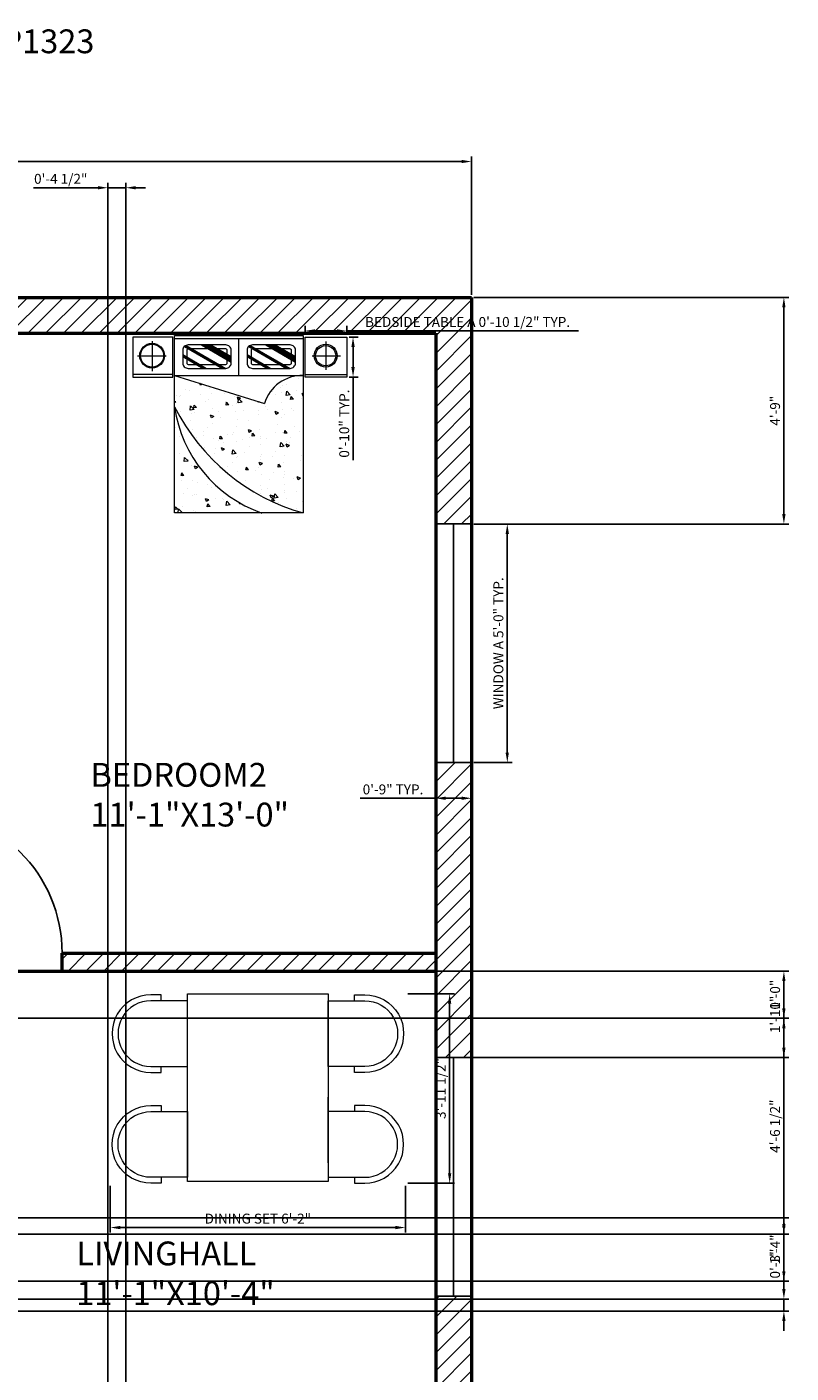
# Model space of a CAD drawing. Units: inches. Extents: x 3064 to 3516, y 2736 to 3280.
# Tile 5 of 5: x 3324 to 3516, y 2941 to 3280. Entities that reach past the tile are written whole.
import ezdxf

# ---------------------------------------------------------------- set-up
doc = ezdxf.new("R2010")
doc.units = ezdxf.units.IN
for name, color, linetype, lineweight in [('A-ANNO-DIMS', 2, 'Continuous', 18), ('A-ANNO-TEXT', 7, 'Continuous', 25), ('A-AREA-IDEN', 6, 'Continuous', 25), ('A-DOOR', 3, 'Continuous', 25), ('A-FURN', 8, 'Continuous', 18), ('A-FURN-PATT', 9, 'Continuous', 13), ('A-GLAZ', 5, 'Continuous', 25), ('A-WALL', 7, 'Continuous', 50), ('A-WALL-PATT', 8, 'Continuous', 13)]:
    doc.layers.add(name, color=color, linetype=linetype, lineweight=lineweight)
doc.styles.get("Standard").update_dxf_attribs({"font": 'arial.ttf'})
doc.dimstyles.new('ISO-25', dxfattribs={"dimtxt": 2.5, "dimasz": 2.5, "dimexe": 1.25, "dimexo": 0.625, "dimtad": 1, "dimlunit": 3, "dimtxsty": 'Standard', "dimcen": 2.5, "dimadec": 0, "dimazin": 0, "dimtfac": 1, "dimtmove": 0, "dimatfit": 3, "dimfxl": 1, "dimarcsym": 0})

# ---------------------------------------------------------------- blocks, each defined once
blk = doc.blocks.new('*D3')
at = {"layer": 'A-ANNO-DIMS', "color": 0, "lineweight": -2, "transparency": 16777216}
for p, q in [((3147.2, 3213.35), (3147.2, 3246.96)), ((3149.7, 3245.71), (3432.9, 3245.71)), ((3435.4, 3212.14), (3435.4, 3246.96))]:
    blk.add_line(p, q, dxfattribs=at)
at = {"layer": 'A-ANNO-DIMS', "color": 0, "transparency": 16777216}
for points in [[(3149.7, 3246.13), (3149.7, 3245.3), (3147.2, 3245.71)], [(3432.9, 3246.13), (3432.9, 3245.3), (3435.4, 3245.71)]]:
    blk.add_solid(points, dxfattribs=at)
at = {"layer": 'Defpoints', "color": 0, "transparency": 16777216}
for p in [(3435.4, 3245.71), (3147.2, 3212.72), (3435.4, 3211.51)]:
    blk.add_point(p, dxfattribs=at)
at = {"layer": 'A-ANNO-DIMS', "color": 0, "transparency": 16777216, "insert": (3291.3, 3249.4), "char_height": 6, "attachment_point": 5}
blk.add_mtext('24\'-0.2"', dxfattribs=at)
blk = doc.blocks.new('4 Person Square 02')
for p, q in [((450, 1104.5), (450, 683.9)), ((-450, 119.2), (-450, 539.9)), ((450, 119.2), (450, 539.9)), ((450, 119.2), (450, 539.9))]:
    blk.add_line(p, q)
for points in [[(-617.2, 1155.3), (-617.2, 1193.5), (-683.2, 1193.5, 1.001343), (-683.2, 697), (-617.2, 697), (-617.2, 735.3)], [(617.2, 1155.3), (617.2, 1193.5), (683.2, 1193.5, -1.001343), (683.2, 697), (617.2, 697), (617.2, 735.3)], [(-617.2, 27.3), (-617.2, -10.9), (-683.2, -10.9, -1.001343), (-683.2, 485.6), (-617.2, 485.6), (-617.2, 447.3)], [(617.2, 27.3), (617.2, -10.9), (683.2, -10.9, 1.001343), (683.2, 485.6), (617.2, 485.6), (617.2, 447.3)]]:
    blk.add_lwpolyline(points, format="xyb")
for points in [[(-450, 735.3), (-450, 1155.3), (-617.2, 1155.3), (-683.2, 1155.3, 1.001587), (-683.2, 735.3)], [(450, 735.3), (450, 1155.3), (617.2, 1155.3), (683.2, 1155.3, -1.001587), (683.2, 735.3)], [(-450, 447.3), (-450, 27.3), (-617.2, 27.3), (-683.2, 27.3, -1.001587), (-683.2, 447.3)], [(450, 447.3), (450, 27.3), (617.2, 27.3), (683.2, 27.3, 1.001587), (683.2, 447.3)]]:
    blk.add_lwpolyline(points, format="xyb", close=True)
blk.add_lwpolyline([(450, 0), (-450, 0), (-450, 1200), (450, 1200)], close=True)
blk = doc.blocks.new('DOOR-SWING-36IN')
for p, q in [((-1, -4.5), (-1, 36)), ((0, 0), (0, 36))]:
    blk.add_line(p, q)
blk.add_arc((0, 0), 36, 90, 180)
blk = doc.blocks.new('WIN-60IN')
for p, q in [((0, 60), (0, 0)), ((9, 60), (0, 60)), ((4.5, 60), (4.5, 0)), ((9, 0), (9, 60)), ((0, 0), (9, 0))]:
    blk.add_line(p, q)
blk = doc.blocks.new('BEDSIDE-TABLE-A')
for p, q in [((0, 0), (0, 10.49)), ((0, 10.49), (10.04, 10.49)), ((9.38, 0), (9.38, 10.49)), ((10.04, 10.49), (10.04, 0)), ((4.67, 1.81), (4.67, 8.9)), ((1.1, 5.18), (8.23, 5.18)), ((10.04, 0), (0, 0))]:
    blk.add_line(p, q)
for radius in [2.89, 2.54]:
    blk.add_circle((4.67, 5.18), radius)
blk = doc.blocks.new('BEDSIDE-TABLE-B')
for p, q in [((10.04, 10.04), (0, 10.04)), ((0, 10.04), (0, 0)), ((4.67, 1.21), (4.67, 8.43)), ((9.34, 0), (9.34, 10.04)), ((10.04, 0), (10.04, 10.04)), ((1.04, 4.86), (8.55, 4.86)), ((0, 0), (10.04, 0))]:
    blk.add_line(p, q)
for radius in [3.11, 2.89]:
    blk.add_circle((4.67, 4.86), radius)
blk = doc.blocks.new('BED-FRAME-AND-COVER')
for p, q in [((0, 32.36), (44.63, 32.36)), ((0, 0), (0, 32.36)), ((0.73, 0), (0.73, 32.36)), ((10.02, 0), (10.02, 32.36)), ((44.63, 32.36), (44.63, 0)), ((10.02, 0), (17.09, 22.61)), ((10.02, 16.18), (0.73, 16.18)), ((44.63, 0), (0, 0))]:
    blk.add_line(p, q)
for centre, radius, start, end in [((20, 32.16), 9.98, 178.8468, 253.0453), ((-5.57, 46.57), 52.17, 296.7955, 344.1914), ((13.16, 33.03), 33.38, 278.2583, 340.5572)]:
    blk.add_arc(centre, radius, start, end)
blk = doc.blocks.new('*D19')
at = {"layer": 'A-ANNO-DIMS', "color": 0, "lineweight": -2, "transparency": 16777216}
for p, q in [((3436.02, 3154.51), (3445.65, 3154.51)), ((3444.4, 3152.01), (3444.4, 3097.01)), ((3436.02, 3094.51), (3445.65, 3094.51))]:
    blk.add_line(p, q, dxfattribs=at)
at = {"layer": 'A-ANNO-DIMS', "color": 0, "transparency": 16777216}
for points in [[(3443.98, 3152.01), (3444.81, 3152.01), (3444.4, 3154.51)], [(3443.98, 3097.01), (3444.81, 3097.01), (3444.4, 3094.51)]]:
    blk.add_solid(points, dxfattribs=at)
at = {"layer": 'Defpoints', "color": 0, "transparency": 16777216}
for p in [(3435.4, 3154.51), (3435.4, 3094.51), (3444.4, 3094.51)]:
    blk.add_point(p, dxfattribs=at)
at = {"layer": 'A-ANNO-DIMS', "color": 0, "transparency": 16777216, "insert": (3442.48, 3124.51), "char_height": 2.5, "attachment_point": 5, "rotation": 90}
blk.add_mtext('WINDOW A 5\'-0" TYP.', dxfattribs=at)
blk = doc.blocks.new('*D20')
at = {"layer": 'A-ANNO-DIMS', "color": 0, "lineweight": -2, "transparency": 16777216}
for p, q in [((3426.4, 3093.89), (3426.4, 3084.26)), ((3435.4, 3093.89), (3435.4, 3084.26)), ((3426.4, 3085.51), (3407.41, 3085.51)), ((3432.9, 3085.51), (3428.9, 3085.51))]:
    blk.add_line(p, q, dxfattribs=at)
at = {"layer": 'A-ANNO-DIMS', "color": 0, "transparency": 16777216}
for points in [[(3428.9, 3085.93), (3428.9, 3085.1), (3426.4, 3085.51)], [(3432.9, 3085.93), (3432.9, 3085.1), (3435.4, 3085.51)]]:
    blk.add_solid(points, dxfattribs=at)
at = {"layer": 'Defpoints', "color": 0, "transparency": 16777216}
for p in [(3426.4, 3094.51), (3435.4, 3094.51), (3426.4, 3085.51)]:
    blk.add_point(p, dxfattribs=at)
at = {"layer": 'A-ANNO-DIMS', "color": 0, "transparency": 16777216, "insert": (3415.65, 3087.42), "char_height": 2.5, "attachment_point": 5}
blk.add_mtext('0\'-9" TYP.', dxfattribs=at)
blk = doc.blocks.new('*D25')
at = {"layer": 'A-ANNO-DIMS', "color": 0, "lineweight": -2, "transparency": 16777216}
for p, q in [((3393.53, 3202.15), (3393.53, 3204.35)), ((3404.02, 3202.15), (3404.02, 3204.35)), ((3396.03, 3203.1), (3401.52, 3203.1)), ((3404.02, 3203.1), (3462.3, 3203.1))]:
    blk.add_line(p, q, dxfattribs=at)
at = {"layer": 'A-ANNO-DIMS', "color": 0, "transparency": 16777216}
for points in [[(3396.03, 3203.51), (3396.03, 3202.68), (3393.53, 3203.1)], [(3401.52, 3203.51), (3401.52, 3202.68), (3404.02, 3203.1)]]:
    blk.add_solid(points, dxfattribs=at)
at = {"layer": 'Defpoints', "color": 0, "transparency": 16777216}
for p in [(3393.53, 3201.52), (3404.02, 3203.1), (3404.02, 3201.52)]:
    blk.add_point(p, dxfattribs=at)
at = {"layer": 'A-ANNO-DIMS', "color": 0, "transparency": 16777216, "insert": (3434.41, 3205.02), "char_height": 2.5, "attachment_point": 5}
blk.add_mtext('BEDSIDE TABLE A 0\'-10 1/2" TYP.', dxfattribs=at)
blk = doc.blocks.new('*D26')
at = {"layer": 'A-ANNO-DIMS', "color": 0, "lineweight": -2, "transparency": 16777216}
for p, q in [((3404.64, 3201.52), (3406.84, 3201.52)), ((3405.59, 3199.02), (3405.59, 3193.98)), ((3404.64, 3191.48), (3406.84, 3191.48)), ((3405.59, 3191.48), (3405.59, 3170.55))]:
    blk.add_line(p, q, dxfattribs=at)
at = {"layer": 'A-ANNO-DIMS', "color": 0, "transparency": 16777216}
for points in [[(3405.17, 3199.02), (3406.01, 3199.02), (3405.59, 3201.52)], [(3405.17, 3193.98), (3406.01, 3193.98), (3405.59, 3191.48)]]:
    blk.add_solid(points, dxfattribs=at)
at = {"layer": 'Defpoints', "color": 0, "transparency": 16777216}
for p in [(3404.02, 3201.52), (3404.02, 3191.48), (3405.59, 3191.48)]:
    blk.add_point(p, dxfattribs=at)
at = {"layer": 'A-ANNO-DIMS', "color": 0, "transparency": 16777216, "insert": (3403.69, 3179.77), "char_height": 2.5, "attachment_point": 5, "rotation": 90}
blk.add_mtext('0\'-10" TYP.', dxfattribs=at)
blk = doc.blocks.new('*D35')
at = {"layer": 'A-ANNO-DIMS', "color": 0, "lineweight": -2, "transparency": 16777216}
for p, q in [((3344.51, 2988.02), (3344.51, 2976.26)), ((3418.76, 2988.02), (3418.76, 2976.26)), ((3347.01, 2977.51), (3416.26, 2977.51))]:
    blk.add_line(p, q, dxfattribs=at)
at = {"layer": 'A-ANNO-DIMS', "color": 0, "transparency": 16777216}
for points in [[(3347.01, 2977.93), (3347.01, 2977.09), (3344.51, 2977.51)], [(3416.26, 2977.93), (3416.26, 2977.09), (3418.76, 2977.51)]]:
    blk.add_solid(points, dxfattribs=at)
at = {"layer": 'Defpoints', "color": 0, "transparency": 16777216}
for p in [(3344.51, 2988.65), (3418.76, 2988.65), (3418.76, 2977.51)]:
    blk.add_point(p, dxfattribs=at)
at = {"layer": 'A-ANNO-DIMS', "color": 0, "transparency": 16777216, "insert": (3381.64, 2979.43), "char_height": 2.5, "attachment_point": 5}
blk.add_mtext('DINING SET 6\'-2"', dxfattribs=at)
blk = doc.blocks.new('*D36')
at = {"layer": 'A-ANNO-DIMS', "color": 0, "lineweight": -2, "transparency": 16777216}
for p, q in [((3419.38, 3036.32), (3431.15, 3036.32)), ((3429.9, 2991.15), (3429.9, 3033.82)), ((3419.38, 2988.65), (3431.15, 2988.65))]:
    blk.add_line(p, q, dxfattribs=at)
at = {"layer": 'A-ANNO-DIMS', "color": 0, "transparency": 16777216}
for points in [[(3429.48, 3033.82), (3430.31, 3033.82), (3429.9, 3036.32)], [(3429.48, 2991.15), (3430.31, 2991.15), (3429.9, 2988.65)]]:
    blk.add_solid(points, dxfattribs=at)
at = {"layer": 'Defpoints', "color": 0, "transparency": 16777216}
for p in [(3418.76, 3036.32), (3429.9, 3036.32), (3418.76, 2988.65)]:
    blk.add_point(p, dxfattribs=at)
at = {"layer": 'A-ANNO-DIMS', "color": 0, "transparency": 16777216, "insert": (3427.98, 3012.49), "char_height": 2.5, "attachment_point": 5, "rotation": 90}
blk.add_mtext('3\'-11 1/2"', dxfattribs=at)
blk = doc.blocks.new('*D41')
at = {"layer": 'A-ANNO-DIMS', "color": 0, "lineweight": -2, "transparency": 16777216}
for p, q in [((3427.02, 3042.01), (3515.25, 3042.01)), ((3514, 3022.76), (3514, 3039.51)), ((3427.02, 3020.26), (3515.25, 3020.26))]:
    blk.add_line(p, q, dxfattribs=at)
at = {"layer": 'A-ANNO-DIMS', "color": 0, "transparency": 16777216}
for points in [[(3513.58, 3039.51), (3514.41, 3039.51), (3514, 3042.01)], [(3513.58, 3022.76), (3514.41, 3022.76), (3514, 3020.26)]]:
    blk.add_solid(points, dxfattribs=at)
at = {"layer": 'Defpoints', "color": 0, "transparency": 16777216}
for p in [(3426.4, 3042.01), (3514, 3042.01), (3426.4, 3020.26)]:
    blk.add_point(p, dxfattribs=at)
at = {"layer": 'A-ANNO-DIMS', "color": 0, "transparency": 16777216, "insert": (3512.1, 3031.14), "char_height": 2.5, "attachment_point": 5, "rotation": 90}
blk.add_mtext('1\'-10"', dxfattribs=at)
blk = doc.blocks.new('*D42')
at = {"layer": 'A-ANNO-DIMS', "color": 0, "lineweight": -2, "transparency": 16777216}
for p, q in [((3436.02, 3211.51), (3515.25, 3211.51)), ((3514, 3157.01), (3514, 3209.01)), ((3436.02, 3154.51), (3515.25, 3154.51))]:
    blk.add_line(p, q, dxfattribs=at)
at = {"layer": 'A-ANNO-DIMS', "color": 0, "transparency": 16777216}
for points in [[(3513.58, 3209.01), (3514.41, 3209.01), (3514, 3211.51)], [(3513.58, 3157.01), (3514.41, 3157.01), (3514, 3154.51)]]:
    blk.add_solid(points, dxfattribs=at)
at = {"layer": 'Defpoints', "color": 0, "transparency": 16777216}
for p in [(3435.4, 3211.51), (3514, 3211.51), (3435.4, 3154.51)]:
    blk.add_point(p, dxfattribs=at)
at = {"layer": 'A-ANNO-DIMS', "color": 0, "transparency": 16777216, "insert": (3512.1, 3183.01), "char_height": 2.5, "attachment_point": 5, "rotation": 90}
blk.add_mtext('4\'-9"', dxfattribs=at)
blk = doc.blocks.new('*D44')
at = {"layer": 'A-ANNO-DIMS', "color": 0, "lineweight": -2, "transparency": 16777216}
for p, q in [((3341.4, 3239.11), (3325.18, 3239.11)), ((3343.9, 2921.14), (3343.9, 3240.36)), ((3348.4, 3239.11), (3343.9, 3239.11)), ((3348.4, 2921.14), (3348.4, 3240.36)), ((3350.9, 3239.11), (3353.4, 3239.11))]:
    blk.add_line(p, q, dxfattribs=at)
at = {"layer": 'A-ANNO-DIMS', "color": 0, "transparency": 16777216}
for points in [[(3341.4, 3239.53), (3341.4, 3238.7), (3343.9, 3239.11)], [(3350.9, 3239.53), (3350.9, 3238.7), (3348.4, 3239.11)]]:
    blk.add_solid(points, dxfattribs=at)
at = {"layer": 'Defpoints', "color": 0, "transparency": 16777216}
for p in [(3343.9, 3239.11), (3343.9, 2920.51), (3348.4, 2920.51)]:
    blk.add_point(p, dxfattribs=at)
at = {"layer": 'A-ANNO-DIMS', "color": 0, "transparency": 16777216, "insert": (3332.04, 3241.03), "char_height": 2.5, "attachment_point": 5}
blk.add_mtext('0\'-4 1/2"', dxfattribs=at)
blk = doc.blocks.new('*D51')
at = {"layer": 'A-ANNO-DIMS', "color": 0, "lineweight": -2, "transparency": 16777216}
for p, q in [((3193.71, 3030.16), (3515.25, 3030.16)), ((3514, 3027.66), (3514, 2978.37)), ((3193.71, 2975.87), (3515.25, 2975.87))]:
    blk.add_line(p, q, dxfattribs=at)
at = {"layer": 'A-ANNO-DIMS', "color": 0, "transparency": 16777216}
for points in [[(3513.58, 3027.66), (3514.41, 3027.66), (3514, 3030.16)], [(3513.58, 2978.37), (3514.41, 2978.37), (3514, 2975.87)]]:
    blk.add_solid(points, dxfattribs=at)
at = {"layer": 'Defpoints', "color": 0, "transparency": 16777216}
for p in [(3193.09, 3030.16), (3193.09, 2975.87), (3514, 2975.87)]:
    blk.add_point(p, dxfattribs=at)
at = {"layer": 'A-ANNO-DIMS', "color": 0, "transparency": 16777216, "insert": (3512.08, 3003.01), "char_height": 2.5, "attachment_point": 5, "rotation": 90}
blk.add_mtext('4\'-6 1/2"', dxfattribs=at)
blk = doc.blocks.new('*D55')
at = {"layer": 'A-ANNO-DIMS', "color": 0, "lineweight": -2, "transparency": 16777216}
for p, q in [((3280.03, 2979.98), (3515.25, 2979.98)), ((3514, 2966.51), (3514, 2977.48)), ((3280.03, 2964.01), (3515.25, 2964.01))]:
    blk.add_line(p, q, dxfattribs=at)
at = {"layer": 'A-ANNO-DIMS', "color": 0, "transparency": 16777216}
for points in [[(3513.58, 2977.48), (3514.41, 2977.48), (3514, 2979.98)], [(3513.58, 2966.51), (3514.41, 2966.51), (3514, 2964.01)]]:
    blk.add_solid(points, dxfattribs=at)
at = {"layer": 'Defpoints', "color": 0, "transparency": 16777216}
for p in [(3279.41, 2979.98), (3514, 2979.98), (3279.41, 2964.01)]:
    blk.add_point(p, dxfattribs=at)
at = {"layer": 'A-ANNO-DIMS', "color": 0, "transparency": 16777216, "insert": (3512.12, 2972), "char_height": 2.5, "attachment_point": 5, "rotation": 90}
blk.add_mtext('1\'-4"', dxfattribs=at)
blk = doc.blocks.new('*D56')
at = {"layer": 'A-ANNO-DIMS', "color": 0, "lineweight": -2, "transparency": 16777216}
for p, q in [((3157.52, 3042.01), (3515.25, 3042.01)), ((3514, 3032.66), (3514, 3039.51)), ((3193.71, 3030.16), (3515.25, 3030.16))]:
    blk.add_line(p, q, dxfattribs=at)
at = {"layer": 'A-ANNO-DIMS', "color": 0, "transparency": 16777216}
for points in [[(3513.58, 3039.51), (3514.41, 3039.51), (3514, 3042.01)], [(3513.58, 3032.66), (3514.41, 3032.66), (3514, 3030.16)]]:
    blk.add_solid(points, dxfattribs=at)
at = {"layer": 'Defpoints', "color": 0, "transparency": 16777216}
for p in [(3156.9, 3042.01), (3514, 3042.01), (3193.09, 3030.16)]:
    blk.add_point(p, dxfattribs=at)
at = {"layer": 'A-ANNO-DIMS', "color": 0, "transparency": 16777216, "insert": (3512.1, 3036.09), "char_height": 2.5, "attachment_point": 5, "rotation": 90}
blk.add_mtext('1\'-0"', dxfattribs=at)
blk = doc.blocks.new('*D59')
at = {"layer": 'A-ANNO-DIMS', "color": 0, "lineweight": -2, "transparency": 16777216}
for p, q in [((3514, 2962.01), (3514, 2972.41)), ((3289.52, 2959.51), (3515.25, 2959.51)), ((3514, 2956.51), (3514, 2959.51)), ((3289.52, 2956.51), (3515.25, 2956.51)), ((3514, 2954.01), (3514, 2951.51))]:
    blk.add_line(p, q, dxfattribs=at)
at = {"layer": 'A-ANNO-DIMS', "color": 0, "transparency": 16777216}
for points in [[(3513.58, 2962.01), (3514.41, 2962.01), (3514, 2959.51)], [(3513.58, 2954.01), (3514.41, 2954.01), (3514, 2956.51)]]:
    blk.add_solid(points, dxfattribs=at)
at = {"layer": 'Defpoints', "color": 0, "transparency": 16777216}
for p in [(3288.9, 2959.51), (3514, 2959.51), (3288.9, 2956.51)]:
    blk.add_point(p, dxfattribs=at)
at = {"layer": 'A-ANNO-DIMS', "color": 0, "transparency": 16777216, "insert": (3512.09, 2968.46), "char_height": 2.5, "attachment_point": 5, "rotation": 90}
blk.add_mtext('0\'-3"', dxfattribs=at)

msp = doc.modelspace()

# ---------------------------------------------------------------- hatches: boundary and pattern name
at = {"layer": 'A-FURN-PATT'}
h = msp.add_hatch(dxfattribs=at)
h.set_pattern_fill('ANSI31', color=256, scale=0.0702842104, angle=105.041628, style=0)
h.paths.add_polyline_path([(3368.824, 3193.671), (3368.744, 3193.671), (3368.297, 3193.671), (3367.85, 3193.671), (3367.77, 3193.671), (3362.743, 3196.569), (3362.743, 3196.615), (3362.743, 3196.873), (3362.743, 3197.13), (3362.743, 3197.177)])
h = msp.add_hatch(dxfattribs=at)
h.set_pattern_fill('ANSI31', color=256, scale=0.0702837215, angle=105.041628, style=0)
h.paths.add_polyline_path([(3373.678, 3193.672), (3373.597, 3193.672), (3373.151, 3193.671), (3372.704, 3193.671), (3372.623, 3193.671), (3363.114, 3199.152), (3363.148, 3199.179), (3363.333, 3199.33), (3363.564, 3199.455), (3363.605, 3199.477)])
h = msp.add_hatch(dxfattribs=at)
h.set_pattern_fill('ANSI31', color=256, scale=0.0702842573, angle=105.041628, style=0)
h.paths.add_polyline_path([(3374.922, 3195.827), (3374.922, 3195.78), (3374.922, 3195.523), (3374.922, 3195.265), (3374.922, 3195.219), (3367.392, 3199.559), (3367.472, 3199.559), (3367.919, 3199.559), (3368.366, 3199.559), (3368.447, 3199.559)])
h = msp.add_hatch(dxfattribs=at)
h.set_pattern_fill('ANSI31', color=256, scale=0.0702851062, angle=105.041628, style=0)
h.paths.add_polyline_path([(3374.922, 3196.662), (3374.922, 3196.615), (3374.922, 3196.358), (3374.922, 3196.1), (3374.922, 3196.054), (3368.84, 3199.559), (3368.921, 3199.559), (3369.368, 3199.559), (3369.814, 3199.559), (3369.895, 3199.559)])
h = msp.add_hatch(dxfattribs=at)
h.set_pattern_fill('ANSI31', color=256, scale=0.0702849307, angle=105.041628, style=0)
h.paths.add_polyline_path([(3385.003, 3193.671), (3384.923, 3193.671), (3384.476, 3193.671), (3384.029, 3193.671), (3383.948, 3193.671), (3378.921, 3196.569), (3378.921, 3196.615), (3378.921, 3196.873), (3378.921, 3197.13), (3378.921, 3197.177)])
h = msp.add_hatch(dxfattribs=at)
h.set_pattern_fill('ANSI31', color=256, scale=0.0702844423, angle=105.041628, style=0)
h.paths.add_polyline_path([(3389.856, 3193.672), (3389.776, 3193.672), (3389.329, 3193.671), (3388.882, 3193.671), (3388.802, 3193.671), (3379.293, 3199.152), (3379.326, 3199.179), (3379.512, 3199.33), (3379.742, 3199.455), (3379.784, 3199.477)])
h = msp.add_hatch(dxfattribs=at)
h.set_pattern_fill('ANSI31', color=256, scale=0.0702849767, angle=105.041628, style=0)
h.paths.add_polyline_path([(3391.101, 3195.827), (3391.101, 3195.78), (3391.101, 3195.523), (3391.101, 3195.265), (3391.101, 3195.219), (3383.571, 3199.559), (3383.651, 3199.559), (3384.098, 3199.559), (3384.545, 3199.559), (3384.625, 3199.559)])
h = msp.add_hatch(dxfattribs=at)
h.set_pattern_fill('ANSI31', color=256, scale=0.070285824, angle=105.041628, style=0)
h.paths.add_polyline_path([(3391.101, 3196.662), (3391.101, 3196.615), (3391.101, 3196.358), (3391.101, 3196.1), (3391.101, 3196.054), (3385.019, 3199.559), (3385.099, 3199.559), (3385.546, 3199.559), (3385.993, 3199.559), (3386.074, 3199.559)])
h = msp.add_hatch(dxfattribs=at)
h.set_pattern_fill('AR-CONC', color=256, scale=0.044631, angle=360, style=0)
h.set_pattern_definition([(130, (3774.2995, 669.116), (-8.131058, -0.711375), [0.850218, -9.352396]), (185, (3774.2995, 669.116), (1.572917, 8.527021), [0.680174, -7.481917]), (79.549, (3773.622, 669.057), (-6.55817, 7.815608), [0.722574, -7.94831]), (133.8158, (3774.299, 671.383), (-12.09849, -1.876385), [1.275327, -14.028594]), (83.3644, (3773.291, 671.227), (-10.595554, 11.042814), [1.08386, -11.922464]), (188.816, (3774.3, 671.383), (-10.59557, 11.042795), [1.02026, -11.222875]), (159, (3773.166, 670.8164), (-6.766702, -4.564198), [0.850218, -9.352396]), (214, (3773.166, 670.816), (-2.758277, 8.220467), [0.680174, -7.481917]), (108.5486, (3772.602, 670.436), (-9.52496, 3.656287), [0.722574, -7.94831]), (142.5, (3774.2995, 669.116), (-0.137847, 3.7737637), [0, -7.391227, 0, -7.595279, 0, -7.510257]), (172.5, (3774.2995, 669.116), (-2.982219, 4.471145), [0, -4.330443, 0, -7.221183, 0, -2.8624]), (212.5, (3776.8274, 669.116), (-6.0515243, -0.2556787), [0, -2.834059, 0, -8.842265, 0, -11.733006]), (222.5, (3777.961, 669.116), (-6.611132, 1.134806), [0, -3.684277, 0, -5.872171, 0, -8.332134])])
edge = h.paths.add_edge_path()
edge.add_ellipse((3392.844, 3181.915), major_axis=(7.055, -7.055), ratio=1, start_angle=136.15316, end_angle=208.04534, ccw=False)
edge.add_line((3392.643, 3191.891), (3393.044, 3191.891))
edge.add_line((3393.044, 3191.891), (3393.044, 3157.28))
edge.add_ellipse((3407.258, 3207.48), major_axis=(36.892, -36.892), ratio=1, start_angle=251.7955, end_angle=299.1914, ccw=False)
edge.add_line((3360.687, 3183.96), (3360.687, 3191.891))
edge.add_line((3360.687, 3191.891), (3383.3, 3184.825))
edge = h.paths.add_edge_path()
edge.add_line((3382.608, 3157.28), (3360.687, 3157.28))
edge.add_line((3360.687, 3157.28), (3360.687, 3183.96))
edge.add_ellipse((3393.718, 3188.754), major_axis=(-23.601, -23.601), ratio=1, start_angle=323.25827, end_angle=385.55722)
at = {"layer": 'A-WALL-PATT'}
h = msp.add_hatch(dxfattribs=at)
h.set_pattern_fill('ANSI31', color=256)
h.paths.add_polyline_path([(3156.897, 2985.015), (3147.897, 2985.015), (3147.897, 2923.515), (3156.897, 2923.515)])
h.paths.add_polyline_path([(3156.897, 2863.515), (3147.897, 2863.515), (3147.897, 2812.515), (3156.897, 2812.515)])
h.paths.add_polyline_path([(3293.397, 2778.015), (3239.397, 2778.015), (3239.397, 2780.015), (3234.897, 2780.015), (3234.897, 2778.015), (3156.897, 2778.015), (3156.897, 2788.515), (3147.897, 2788.515), (3147.897, 2769.015), (3293.397, 2769.015)])
h.paths.add_polyline_path([(3369.397, 2778.015), (3343.897, 2778.015), (3344.15, 2769.015), (3369.397, 2769.015)])
h.paths.add_polyline_path([(3435.397, 2788.515), (3426.397, 2788.515), (3426.397, 2778.015), (3405.397, 2778.015), (3405.397, 2769.015), (3435.397, 2769.015)])
h.paths.add_polyline_path([(3435.397, 2960.265), (3426.397, 2960.265), (3426.397, 2812.515), (3435.397, 2812.515)])
h.paths.add_polyline_path([(3435.397, 3094.515), (3426.397, 3094.515), (3426.397, 3020.265), (3435.397, 3020.265)])
h.paths.add_polyline_path([(3435.397, 3211.515), (3147.897, 3211.515), (3147.897, 3154.515), (3156.897, 3154.515), (3156.897, 3202.515), (3426.397, 3202.515), (3426.397, 3154.515), (3435.397, 3154.515)])
h.paths.add_polyline_path([(3293.397, 3202.515), (3288.897, 3202.515), (3288.897, 3046.515), (3285.897, 3046.515), (3285.897, 3042.015), (3296.397, 3042.015), (3296.397, 3046.515), (3293.397, 3046.515)])
h.paths.add_polyline_path([(3426.397, 3046.515), (3332.397, 3046.515), (3332.397, 3042.015), (3426.397, 3042.015)])
h.paths.add_polyline_path([(3249.897, 3046.515), (3156.897, 3046.515), (3156.897, 3042.015), (3249.897, 3042.015)])
h.paths.add_polyline_path([(3156.897, 3094.515), (3147.897, 3094.515), (3147.897, 3021.015), (3156.897, 3021.015)])
h.paths.add_polyline_path([(3293.397, 2964.015), (3156.897, 2964.015), (3156.897, 2959.515), (3288.897, 2959.515), (3288.897, 2956.515), (3293.397, 2956.515)])
h.paths.add_polyline_path([(3249.897, 2827.515), (3156.897, 2827.515), (3156.897, 2823.015), (3234.897, 2823.015), (3234.897, 2816.015), (3239.397, 2816.015), (3239.397, 2823.015), (3249.897, 2823.015)])
h.paths.add_polyline_path([(3293.397, 2920.515), (3288.897, 2920.515), (3288.897, 2827.515), (3285.897, 2827.515), (3285.897, 2823.015), (3293.397, 2823.015), (3293.397, 2856.015), (3305.897, 2856.015), (3305.897, 2860.515), (3293.397, 2860.515)])
h.paths.add_polyline_path([(3348.397, 2920.515), (3343.897, 2920.515), (3343.897, 2860.515), (3341.897, 2860.515), (3341.897, 2856.015), (3343.897, 2856.015), (3343.897, 2778.015), (3348.397, 2778.015), (3348.397, 2823.015), (3350.397, 2823.015), (3350.397, 2827.515), (3348.397, 2827.515)])
h.paths.add_polyline_path([(3426.397, 2827.515), (3386.397, 2827.515), (3386.397, 2823.015), (3426.397, 2823.015)])

# ---------------------------------------------------------------- linework, layer by layer
at = {"layer": 'A-FURN'}
for points in [[(3373.583, 3199.559), (3364.082, 3199.559, 0.4142136), (3362.743, 3198.22), (3362.743, 3195.01, 0.4142136), (3364.082, 3193.671), (3373.583, 3193.671, 0.4142136), (3374.922, 3195.01), (3374.922, 3198.22, 0.4142136)], [(3373.583, 3198.555), (3364.082, 3198.555, 0.4142136), (3363.747, 3198.22), (3363.747, 3195.01, 0.4142136), (3364.082, 3194.676), (3373.583, 3194.676, 0.4142136), (3373.918, 3195.01), (3373.918, 3198.22, 0.4142136)], [(3389.762, 3199.559), (3380.26, 3199.559, 0.4142136), (3378.921, 3198.22), (3378.921, 3195.01, 0.4142136), (3380.26, 3193.671), (3389.762, 3193.671, 0.4142136), (3391.101, 3195.01), (3391.101, 3198.22, 0.4142136)], [(3389.762, 3198.555), (3380.26, 3198.555, 0.4142136), (3379.926, 3198.22), (3379.926, 3195.01, 0.4142136), (3380.26, 3194.676), (3389.762, 3194.676, 0.4142136), (3390.096, 3195.01), (3390.096, 3198.22, 0.4142136)]]:
    msp.add_lwpolyline(points, format="xyb", close=True, dxfattribs=at)
at = {"layer": 'A-WALL'}
for p, q in [((3147.897, 3211.515), (3435.397, 3211.515)), ((3435.397, 3211.515), (3435.397, 2769.015)), ((3156.897, 3202.515), (3426.397, 3202.515)), ((3426.397, 3202.515), (3426.397, 2778.015)), ((3332.397, 3042.015), (3332.397, 3046.515)), ((3332.397, 3046.515), (3426.397, 3046.515)), ((3156.897, 3042.015), (3426.397, 3042.015))]:
    msp.add_line(p, q, dxfattribs=at)

# ---------------------------------------------------------------- block references
at = {"layer": 'A-DOOR', "extrusion": (0, 0, -1), "zscale": -1}
msp.add_blockref('DOOR-SWING-36IN', (-3296.397, 3046.515), dxfattribs=at)
at = {"layer": 'A-FURN'}
for name, p, rotation in [('BEDSIDE-TABLE-B', (3350.164, 3201.524), 269.9999999999973), ('BED-FRAME-AND-COVER', (3360.687, 3201.911), 270.0000000000024), ('BEDSIDE-TABLE-A', (3393.526, 3201.524), 269.999999999995)]:
    msp.add_blockref(name, p, dxfattribs=dict(at, rotation=rotation))
at = {"layer": 'A-FURN', "xscale": 0.0393700787401575, "yscale": 0.0393700787401575, "zscale": 0.0393700787401575}
msp.add_blockref('4 Person Square 02', (3381.636, 2989.08), dxfattribs=at)
at = {"layer": 'A-GLAZ', "rotation": 180}
msp.add_blockref('WIN-60IN', (3435.397, 3154.515), dxfattribs=at)
at = {"layer": 'A-GLAZ'}
msp.add_blockref('WIN-60IN', (3426.397, 2960.265), dxfattribs=at)

# ---------------------------------------------------------------- texts
at = {"layer": 'A-ANNO-TEXT', "insert": (3166.949, 3278.95), "char_height": 6, "attachment_point": 1}
msp.add_mtext_dynamic_manual_height_columns('24X37\\{888sq ft\\}House Plan-West Face-FP1323', width=332.43103, gutter_width=12.5, heights=[0], dxfattribs=at)
at = {"layer": 'A-AREA-IDEN', "char_height": 6, "attachment_point": 1}
for s, insert in [('BEDROOM2\\P11\'-1"X13\'-0"', (3339.527, 3094.403)), ('LIVINGHALL\\P11\'-1"X10\'-4"', (3335.939, 2973.991))]:
    msp.add_mtext(s, dxfattribs=dict(at, insert=insert))

# ---------------------------------------------------------------- dimensions: what is measured, and where the dimension line sits
at = {"layer": 'A-ANNO-DIMS'}
for base, p1, p2, override, picture, middle in [((3435.397, 3245.713), (3147.2, 3212.723), (3435.397, 3211.515), {"dimtxt": 6, "dimclrd": 0, "dimclre": 0, "dimclrt": 0}, '*D3', (3291.299, 3249.402)), ((3343.897, 3239.115), (3348.397, 2920.515), (3343.897, 2920.515), {"dimdec": 1, "dimlfac": 1, "dimrnd": 0, "dimzin": 1, "dimdsep": 46, "dimlunit": 4, "dimfrac": 2}, '*D44', (3332.037, 3241.033))]:
    dim = msp.add_linear_dim(base=base, p1=p1, p2=p2, dimstyle='ISO-25', override=override, dxfattribs=at)
    dim.commit()
    dim.dimension.update_dxf_attribs({"geometry": picture, "text_midpoint": middle})
for base, p1, p2, text, picture, middle in [((3404.018, 3203.098), (3393.526, 3201.524), (3404.018, 3201.524), 'BEDSIDE TABLE A <> TYP.', '*D25', (3434.409, 3205.016)), ((3418.759, 2977.51), (3344.513, 2988.647), (3418.759, 2988.647), 'DINING SET <>', '*D35', (3381.636, 2979.427))]:
    dim = msp.add_linear_dim(base=base, p1=p1, p2=p2, text=text, dimstyle='ISO-25', override={"dimdec": 1, "dimlfac": 1, "dimrnd": 0, "dimzin": 1, "dimdsep": 46, "dimlunit": 4, "dimfrac": 2}, dxfattribs=at)
    dim.commit()
    dim.dimension.update_dxf_attribs({"geometry": picture, "text_midpoint": middle})
for base, p1, p2, picture, middle in [((3513.997, 3211.515), (3435.397, 3154.515), (3435.397, 3211.515), '*D42', (3512.096, 3183.015)), ((3513.997, 3042.015), (3193.09, 3030.159), (3156.897, 3042.015), '*D56', (3512.096, 3036.087)), ((3513.997241, 3042.01493), (3426.397241, 3020.26493), (3426.397241, 3042.01493), '*D41', (3512.095808531, 3031.13993)), ((3429.896, 3036.324), (3418.759, 2988.647), (3418.759, 3036.324), '*D36', (3427.977, 3012.486)), ((3513.997, 2975.87), (3193.09, 3030.159), (3193.09, 2975.87), '*D51', (3512.08, 3003.015)), ((3513.997, 2979.978), (3279.406, 2964.015), (3279.406, 2979.978), '*D55', (3512.117, 2971.997)), ((3513.997, 2959.515), (3288.897, 2956.515), (3288.897, 2959.515), '*D59', (3512.095, 2968.463))]:
    dim = msp.add_linear_dim(base=base, p1=p1, p2=p2, angle=90, dimstyle='ISO-25', override={"dimdec": 1, "dimlfac": 1, "dimrnd": 0, "dimzin": 1, "dimdsep": 46, "dimlunit": 4, "dimfrac": 2}, dxfattribs=at)
    dim.commit()
    dim.dimension.update_dxf_attribs({"geometry": picture, "text_midpoint": middle})
for base, p1, p2, angle, text, picture, middle in [((3405.591, 3191.482), (3404.018, 3201.524), (3404.018, 3191.482), 270, '<> TYP.', '*D26', (3403.69, 3179.767)), ((3444.397, 3094.515), (3435.397, 3154.515), (3435.397, 3094.515), 270, 'WINDOW A <> TYP.', '*D19', (3442.479, 3124.515)), ((3426.397, 3085.515), (3435.397, 3094.515), (3426.397, 3094.515), 180, '<> TYP.', '*D20', (3415.653, 3087.416))]:
    dim = msp.add_linear_dim(base=base, p1=p1, p2=p2, angle=angle, text=text, dimstyle='ISO-25', override={"dimdec": 1, "dimlfac": 1, "dimrnd": 0, "dimzin": 1, "dimdsep": 46, "dimlunit": 4, "dimfrac": 2}, dxfattribs=at)
    dim.commit()
    dim.dimension.update_dxf_attribs({"geometry": picture, "text_midpoint": middle})

doc.saveas('drawing.dxf')
